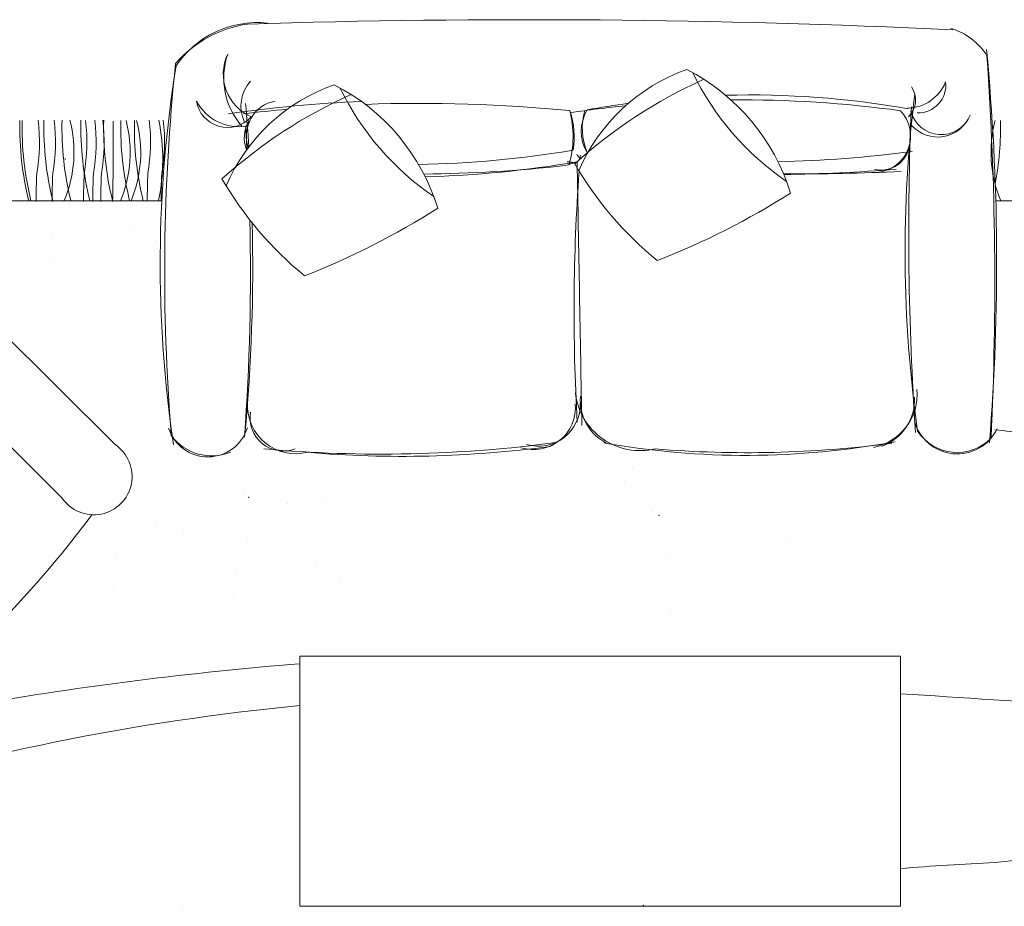
# Model space of a CAD drawing. Units: inches. Extents: x 182 to 1022, y -617 to 111.
# Tile 8 of 33: x 294 to 363, y -278 to -215. Entities that reach past the tile are written whole.
import ezdxf

# ---------------------------------------------------------------- set-up
doc = ezdxf.new("R2010")
doc.units = ezdxf.units.IN
doc.header["$MEASUREMENT"] = 0
doc.layers.add('furniture', color=50, linetype='Continuous', lineweight=15, transparency=0.8)

# ---------------------------------------------------------------- blocks, each defined once
blk = doc.blocks.new('LOUNGE-SEATING-GROUP')
for p, q in [((38.821, 71.99), (38.821, 71.99)), ((22.374, 71.638), (42.714, 51.416)), ((41.949, 71.175), (41.949, 71.175)), ((44.619, 71.402), (44.619, 71.402)), ((25.374, 68.655), (46.023, 68.655)), ((39.146, 68.689), (39.146, 68.689)), ((104.961, 68.655), (107.809, 68.655)), ((38.275, 66.239), (38.275, 66.239)), ((43.998, 66.686), (43.998, 66.686)), ((45.677, 65.873), (45.677, 65.873)), ((38.143, 64.53), (38.143, 64.53)), ((23.811, 62.711), (38.962, 47.665)), ((79.299, 49.738), (79.299, 49.738)), ((79.299, 49.738), (79.299, 49.738)), ((78.687, 48.814), (78.687, 48.814)), ((78.687, 48.814), (78.687, 48.814)), ((51.766, 48.079), (51.766, 48.079)), ((57.565, 47.491), (57.565, 47.491)), ((54.895, 47.264), (54.895, 47.264)), ((80.668, 46.7), (80.668, 46.7)), ((40.731, 45.33), (40.731, 45.33)), ((40.731, 45.33), (40.731, 45.33)), ((45.545, 45.809), (45.545, 45.809)), ((47.546, 45.107), (47.546, 45.107)), ((52.091, 44.778), (52.091, 44.778)), ((90.412, 44.74), (90.412, 44.74)), ((42.774, 43.403), (42.774, 43.403)), ((81.888, 43.615), (81.888, 43.615)), ((56.944, 42.774), (56.944, 42.774)), ((51.221, 42.328), (51.221, 42.328)), ((58.622, 41.962), (58.622, 41.962)), ((42.63, 41.412), (42.63, 41.412)), ((51.089, 40.619), (51.089, 40.619)), ((81.951, 39.421), (81.951, 39.421)), ((55.774, 18.787), (55.774, 36.473)), ((55.774, 36.473), (98.219, 36.473)), ((98.219, 36.473), (98.219, 18.787)), ((47.451, 18.854), (47.451, 18.854)), ((98.219, 18.787), (55.774, 18.787))]:
    blk.add_line(p, q)
for centre, radius, start, end in [((71.794, -550.873), 632.322, 87.2697, 91.787503), ((52.765, 74.335), 6.91, 83.87925, 147.10928), ((53.342, 72.785), 8.453, 98.65495, 138.71038), ((100.543, 76.542), 4.466, 31.88171, 73.96721), ((-54.46, 64.251), 159.482, 355.43246, 5.43098), ((53.655, 77.606), 3.29, 154.87152, 246.7247), ((55.598, 77.332), 5.198, 161.24727, 221.13483), ((-129.185, 62.846), 234.072, 357.31429, 3.93296), ((133.781, 64.161), 87.874, 170.80787, 188.3514), ((189.048, 63.589), 142.823, 174.0627, 184.62528), ((87.466, 65.638), 13.032, 109.45006, 156.76991), ((76.483, 64.92), 14.605, 17.0126, 62.9429), ((101.322, 86.342), 19.767, 205.90051, 235.65125), ((62.538, 64.566), 13.032, 109.45006, 156.76991), ((54.241, 75.334), 2.626, 137.72028, 204.44608), ((51.555, 63.848), 14.605, 17.0126, 62.9429), ((76.393, 85.27), 19.767, 205.90051, 235.65125), ((98.417, 45.727), 34.512, 114.08153, 132.27682), ((98.669, 78.165), 2.966, 271.18396, 337.82163), ((97.614, 75.782), 1.677, 314.39377, 33.58565), ((99.47, 76.821), 1.959, 268.0108, 6.55846), ((73.489, 44.655), 34.512, 114.08153, 132.27682), ((87.642, 12.429), 63.701, 79.94664, 91.59031), ((189.766, 65.051), 91.216, 172.98362, 187.98903), ((51.469, 77.275), 3.389, 207.84326, 279.86837), ((50.666, 76.051), 2.224, 189.29162, 317.62886), ((63.548, -12.927), 88.655, 92.2017, 98.30671), ((-77.454, 64.061), 129.9, 3.71005, 5.06529), ((54.497, 73.237), 2.502, 100.62162, 199.19299), ((64.364, -31.324), 106.862, 84.36393, 92.12187), ((87.048, -6.169), 81.952, 95.77953, 98.52202), ((87.642, 12.429), 63.701, 97.80299, 100.45572), ((87.048, -6.169), 81.952, 82.15508, 90.55852), ((303.256, 66.394), 204.452, 177.50734, 183.9592), ((64.364, -31.324), 106.862, 95.08707, 96.74912), ((67.782, 73.23), 7.3, 344.04794, 14.20605), ((69.169, 73.114), 5.999, 351.53624, 18.34934), ((78.622, 73.558), 2.957, 149.83188, 209.46797), ((80.087, 73.775), 4.352, 163.31083, 202.61636), ((96.334, 73.238), 2.603, 276.1174, 43.1189), ((101.1, 75.541), 2.219, 194.78136, 337.59217), ((100.85, 75.643), 2.488, 222.31343, 337.61024), ((57.542, 73.818), 21.554, 178.63307, 193.85735), ((57.703, 73.818), 21.554, 178.63307, 193.85735), ((24.582, 72.804), 12.794, 349.93491, 6.88295), ((59.241, 73.824), 21.554, 178.63307, 193.85735), ((25.712, 72.807), 12.794, 349.93491, 6.88295), ((60.516, 73.834), 21.554, 178.63307, 193.85735), ((30.979, 72.079), 8.837, 337.30984, 14.86132), ((61.856, 73.831), 21.554, 178.63307, 193.85735), ((27.933, 72.798), 12.794, 349.93491, 6.88295), ((28.587, 72.808), 12.794, 349.93491, 6.88295), ((29.152, 72.809), 12.794, 349.93491, 6.88295), ((63.464, 73.829), 21.554, 178.63307, 193.85735), ((-141.927, 73.02), 184.521, 358.62796, 0.39341), ((34.952, 72.065), 8.837, 337.30984, 14.86132), ((64.672, 73.82), 21.554, 178.63307, 193.85735), ((35.695, 72.056), 8.837, 337.30984, 14.86132), ((65.635, 73.812), 21.554, 178.63307, 193.85735), ((32.435, 72.811), 12.794, 349.93491, 6.88295), ((31.753, 71.547), 14.333, 348.41121, 11.24547), ((33.421, 72.813), 12.794, 349.93491, 6.88295), ((54.088, 73.1), 2.242, 147.73663, 202.23873), ((-105.601, 63.498), 157.885, 3.19084, 3.78915), ((113.459, 72.065), 8.837, 165.13868, 202.69016), ((83.739, 73.82), 21.554, 349.37308, 1.36693), ((96.83, 72.878), 2.062, 257.62255, 350.30943), ((62.879, 144.509), 73.304, 271.00607, 279.60009), ((76.97, 72.854), 1.854, 209.13127, 222.01414), ((211.777, 60.833), 136.621, 175.36553, 175.4784), ((87.421, 161.016), 89.637, 262.72451, 262.77255), ((87.421, 161.016), 89.637, 271.37312, 277.44721), ((63.687, 168.954), 98.418, 270.49489, 276.32914), ((62.388, 148.587), 78.275, 271.64583, 279.52678), ((83.934, 41.266), 31.314, 105.96247, 107.46375), ((90.922, 223.121), 152.575, 263.88721, 264.12153), ((97.264, 84.159), 25.556, 210.30685, 230.5663), ((-1557724.038, -27714.166), 1558047.191, 1.021158169, 1.0218453), ((179.822, 66.058), 142.714, 178.18909, 178.97752), ((180.953, 66.061), 142.714, 178.18909, 178.97752), ((183.173, 66.052), 142.714, 178.18909, 178.97752), ((183.827, 66.062), 142.714, 178.18909, 178.97752), ((184.392, 66.064), 142.714, 178.18909, 178.97752), ((187.675, 66.065), 142.714, 178.18909, 178.97752), ((188.661, 66.067), 142.714, 178.18909, 178.97752), ((211.777, 60.833), 136.621, 175.84252, 183.2873), ((90.922, 223.121), 152.575, 269.63856, 272.76525), ((88.379, 193.19), 122.689, 270.7456, 274.45597), ((72.336, 83.087), 25.556, 210.30685, 230.5663), ((61.136, 115.352), 54.68, 291.33709, 302.41765), ((36.207, 114.281), 54.68, 291.33709, 302.41765), ((-105.601, 63.498), 157.885, 355.80271, 1.38032), ((-77.454, 64.061), 129.9, 354.74224, 1.33354), ((79.824, 55.598), 4.608, 186.58671, 283.45107), ((95.579, 54.982), 3.827, 280.97559, 4.97468), ((55.471, 54.171), 3.397, 177.65794, 284.09744), ((72.278, 54.042), 2.978, 252.93165, 5.10915), ((72.646, 54.256), 2.952, 253.4437, 1.82282), ((78.963, 54.532), 3.365, 174.92344, 245.63742), ((95.685, 54.626), 3.543, 289.82281, 2.49854), ((54.612, 53.317), 2.353, 170.26169, 291.01149), ((102.233, 53.891), 3.128, 194.63788, 334.30948), ((49.285, 53.468), 2.918, 197.71573, 342.84284), ((102.229, 54.191), 3.334, 213.04105, 316.06525), ((219.704, 1090.605), 1044.469, 263.689239, 263.937357), ((49.538, 54.146), 3.523, 216.0678, 292.6723), ((61.571, 143.109), 92.365, 264.82447, 277.71479), ((87.313, 108.916), 58.258, 260.0543, 280.4167), ((87.395, 128.627), 77.782, 265.20718, 277.55097), ((41.215, 49.163), 2.706, 213.6335, 56.3665), ((63.009, 128.803), 78.216, 265.07811, 277.69498), ((-19.252, 91.372), 75.219, 306.60494, 323.33873), ((76.484, -220.38), 257.147, 94.61959, 99.75131), ((-225.395, -5012.463), 5056.639, 86.03178, 86.330686), ((71.513, -132.242), 165.958, 95.44209, 107.47988), ((219.704, -1016.256), 1044.469, 94.698728, 96.310761), ((115.905, -204.233), 226.385, 92.78771, 94.48071)]:
    blk.add_arc(centre, radius, start, end)
for p in [(39.213, 71.597), (52.158, 47.686), (81.153, 46.43), (80.044, 18.85)]:
    blk.add_point(p)

msp = doc.modelspace()

# ---------------------------------------------------------------- block references
at = {"layer": 'furniture'}
msp.add_blockref('LOUNGE-SEATING-GROUP', (257.848, -296.822), dxfattribs=at)

doc.saveas('drawing.dxf')
